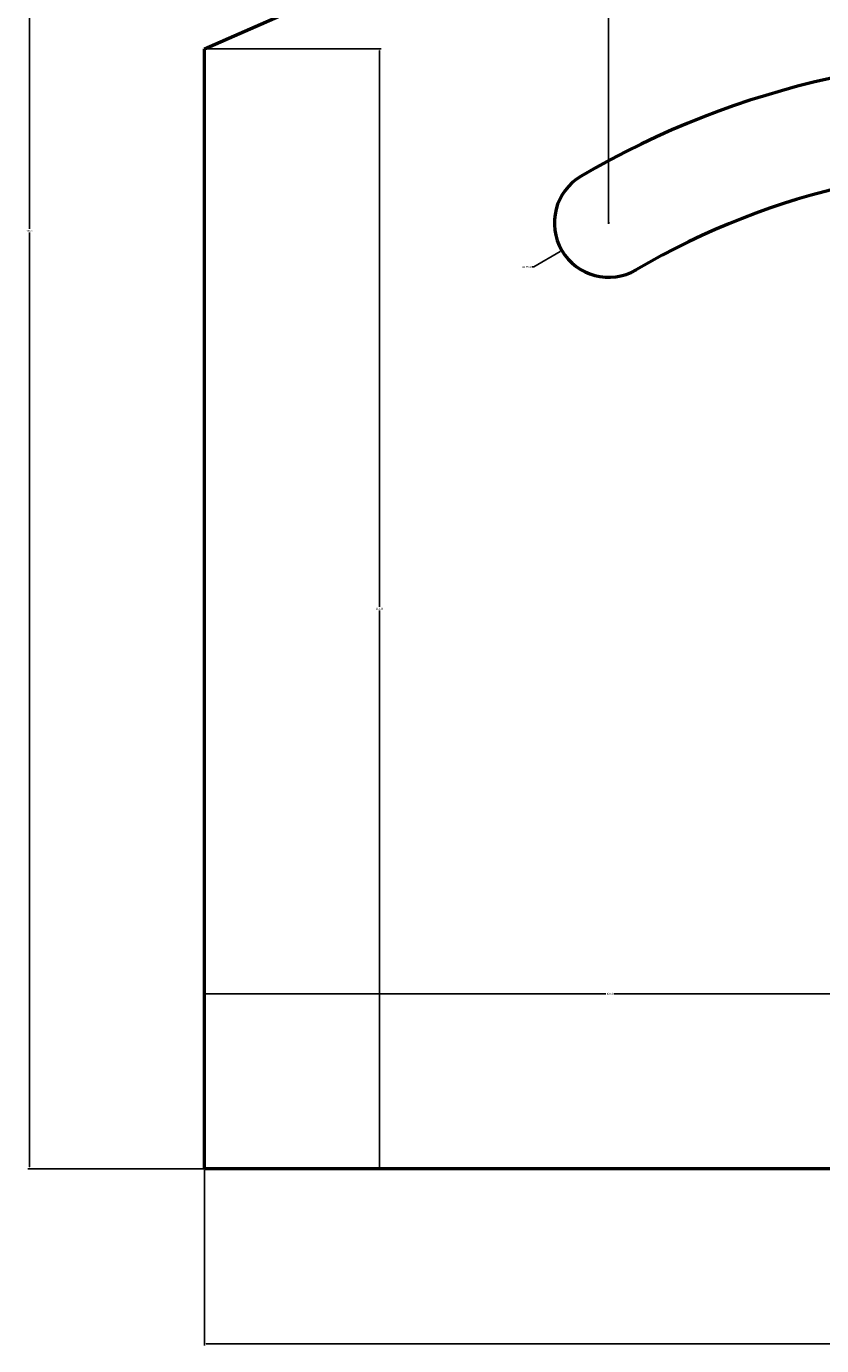
# Model space of a CAD drawing. Units: inches. Extents: x 457 to 775, y 319 to 541.
# Tile 1 of 12: x 457 to 536, y 319 to 450. Entities that reach past the tile are written whole.
import ezdxf

# ---------------------------------------------------------------- set-up
doc = ezdxf.new("R2010")
doc.units = ezdxf.units.IN
doc.header["$MEASUREMENT"] = 0
doc.layers.add('M-DIMS', color=2, linetype='Continuous', lineweight=18)
doc.layers.add('M-OUTL', color=7, linetype='Continuous', lineweight=50)
doc.styles.get("Standard").update_dxf_attribs({"font": 'arial.ttf'})
doc.dimstyles.get("Standard").update_dxf_attribs({"dimtxt": 0.18, "dimasz": 0.18, "dimexe": 0.18, "dimexo": 0.0625, "dimgap": 0.09, "dimtad": 0, "dimtih": 1, "dimtoh": 1, "dimdec": 4, "dimzin": 0, "dimdsep": 46, "dimtxsty": 'Standard', "dimcen": 0.09, "dimadec": 0, "dimazin": 0, "dimtfac": 1, "dimtdec": 4, "dimtofl": 0, "dimtmove": 0, "dimatfit": 3, "dimfxl": 1, "dimtolj": 1, "dimtzin": 0, "dimarcsym": 0})

# ---------------------------------------------------------------- blocks, each defined once
blk = doc.blocks.new('*D2')
at = {"layer": 'Defpoints', "color": 0, "transparency": 16777216}
for p in [(756.93, 375.7), (474.31, 336.7), (756.93, 319.3)]:
    blk.add_point(p, dxfattribs=at)
at = {"layer": 'M-DIMS', "color": 0, "lineweight": -2, "transparency": 16777216}
for p, q in [((756.93, 375.63), (756.93, 319.12)), ((474.31, 336.63), (474.31, 319.12)), ((474.49, 319.3), (615.22, 319.3)), ((756.75, 319.3), (616.01, 319.3))]:
    blk.add_line(p, q, dxfattribs=at)
at = {"layer": 'M-DIMS', "color": 0, "transparency": 16777216}
for points in [[(474.49, 319.33), (474.49, 319.27), (474.31, 319.3)], [(756.75, 319.33), (756.75, 319.27), (756.93, 319.3)]]:
    blk.add_solid(points, dxfattribs=at)
at = {"layer": 'M-DIMS', "color": 0, "transparency": 16777216, "insert": (615.62, 319.3), "char_height": 0.18, "attachment_point": 5}
blk.add_mtext('\\A1;282.6', dxfattribs=at)
blk = doc.blocks.new('*D3')
at = {"layer": 'Defpoints', "color": 0, "transparency": 16777216}
for p in [(456.91, 523.21), (646, 523.21), (474.31, 336.7)]:
    blk.add_point(p, dxfattribs=at)
at = {"layer": 'M-DIMS', "color": 0, "lineweight": -2, "transparency": 16777216}
for p, q in [((645.94, 523.21), (456.73, 523.21)), ((456.91, 523.03), (456.91, 430.14)), ((456.91, 336.88), (456.91, 429.77)), ((474.24, 336.7), (456.73, 336.7))]:
    blk.add_line(p, q, dxfattribs=at)
at = {"layer": 'M-DIMS', "color": 0, "transparency": 16777216}
for points in [[(456.88, 523.03), (456.94, 523.03), (456.91, 523.21)], [(456.88, 336.88), (456.94, 336.88), (456.91, 336.7)]]:
    blk.add_solid(points, dxfattribs=at)
at = {"layer": 'M-DIMS', "color": 0, "transparency": 16777216, "insert": (456.91, 429.95), "char_height": 0.18, "attachment_point": 5}
blk.add_mtext('\\A1;186.5', dxfattribs=at)
blk = doc.blocks.new('*D5')
at = {"layer": 'Defpoints', "color": 0, "transparency": 16777216}
for p in [(474.31, 448.06), (474.31, 336.7), (491.71, 336.7)]:
    blk.add_point(p, dxfattribs=at)
at = {"layer": 'M-DIMS', "color": 0, "lineweight": -2, "transparency": 16777216}
for p, q in [((474.37, 448.06), (491.89, 448.06)), ((491.71, 447.88), (491.71, 392.56)), ((491.71, 336.88), (491.71, 392.2)), ((474.37, 336.7), (491.89, 336.7))]:
    blk.add_line(p, q, dxfattribs=at)
at = {"layer": 'M-DIMS', "color": 0, "transparency": 16777216}
for points in [[(491.68, 447.88), (491.74, 447.88), (491.71, 448.06)], [(491.68, 336.88), (491.74, 336.88), (491.71, 336.7)]]:
    blk.add_solid(points, dxfattribs=at)
at = {"layer": 'M-DIMS', "color": 0, "transparency": 16777216, "insert": (491.71, 392.38), "char_height": 0.18, "attachment_point": 5}
blk.add_mtext('\\A1;111.36', dxfattribs=at)
blk = doc.blocks.new('*D6')
at = {"layer": 'Defpoints', "color": 0, "transparency": 16777216}
for p in [(554.93, 354.1), (474.31, 336.7), (554.93, 336.7)]:
    blk.add_point(p, dxfattribs=at)
at = {"layer": 'M-DIMS', "color": 0, "lineweight": -2, "transparency": 16777216}
for p, q in [((474.31, 336.76), (474.31, 354.28)), ((554.93, 336.76), (554.93, 354.28)), ((474.49, 354.1), (514.23, 354.1)), ((554.75, 354.1), (515.01, 354.1))]:
    blk.add_line(p, q, dxfattribs=at)
at = {"layer": 'M-DIMS', "color": 0, "transparency": 16777216}
for points in [[(474.49, 354.13), (474.49, 354.07), (474.31, 354.1)], [(554.75, 354.13), (554.75, 354.07), (554.93, 354.1)]]:
    blk.add_solid(points, dxfattribs=at)
at = {"layer": 'M-DIMS', "color": 0, "transparency": 16777216, "insert": (514.62, 354.1), "char_height": 0.18, "attachment_point": 5}
blk.add_mtext('\\A1;80.62', dxfattribs=at)
blk = doc.blocks.new('*D16')
at = {"layer": 'Defpoints', "color": 0, "transparency": 16777216}
for p in [(554.93, 540.61), (514.5, 430.73), (554.93, 361.7)]:
    blk.add_point(p, dxfattribs=at)
at = {"layer": 'M-DIMS', "color": 0, "lineweight": -2, "transparency": 16777216}
for p, q in [((514.5, 430.79), (514.5, 540.79)), ((514.68, 540.61), (534.32, 540.61)), ((554.75, 540.61), (535.11, 540.61)), ((554.93, 361.76), (554.93, 540.79))]:
    blk.add_line(p, q, dxfattribs=at)
at = {"layer": 'M-DIMS', "color": 0, "transparency": 16777216}
for points in [[(514.68, 540.64), (514.68, 540.58), (514.5, 540.61)], [(554.75, 540.64), (554.75, 540.58), (554.93, 540.61)]]:
    blk.add_solid(points, dxfattribs=at)
at = {"layer": 'M-DIMS', "color": 0, "transparency": 16777216, "insert": (534.72, 540.61), "char_height": 0.18, "attachment_point": 5}
blk.add_mtext('\\A1;40.43', dxfattribs=at)
blk = doc.blocks.new('*D21')
at = {"layer": 'Defpoints', "color": 0, "transparency": 16777216}
for p in [(514.5, 430.73), (509.84, 428)]:
    blk.add_point(p, dxfattribs=at)
at = {"layer": 'M-DIMS', "color": 0, "lineweight": -2, "transparency": 16777216}
for p, q in [((514.41, 430.73), (514.59, 430.73)), ((514.5, 430.64), (514.5, 430.82)), ((507.05, 426.36), (509.69, 427.91)), ((506.87, 426.36), (507.05, 426.36))]:
    blk.add_line(p, q, dxfattribs=at)
at = {"layer": 'M-DIMS', "color": 0, "transparency": 16777216}
blk.add_solid([(509.67, 427.93), (509.7, 427.88), (509.84, 428)], dxfattribs=at)
at = {"layer": 'M-DIMS', "color": 0, "transparency": 16777216, "insert": (506.33, 426.36), "char_height": 0.18, "attachment_point": 5}
blk.add_mtext('\\A1;2X R5.4', dxfattribs=at)

msp = doc.modelspace()

# ---------------------------------------------------------------- linework, layer by layer
at = {"layer": 'M-OUTL'}
for p, q in [((474.306, 448.059), (646.001, 523.213)), ((474.306, 336.696), (474.306, 448.059)), ((554.931, 336.696), (474.306, 336.696))]:
    msp.add_line(p, q, dxfattribs=at)
for centre, radius, start, end in [((554.931, 361.696), 85.4, 49.61848, 120.35555), ((554.931, 361.696), 74.6, 49.61848, 120.35555), ((514.502, 430.729), 5.4, 120.35555, 300.35555)]:
    msp.add_arc(centre, radius, start, end, dxfattribs=at)

# ---------------------------------------------------------------- dimensions: what is measured, and where the dimension line sits
at = {"layer": 'M-DIMS'}
for base, p1, p2, override, picture, middle in [((554.931, 540.613), (514.502, 430.729), (554.931, 361.696), {"dimdec": 2, "dimlfac": 1, "dimrnd": 0, "dimzin": 0, "dimdsep": 46, "dimlunit": 2}, '*D16', (534.716, 540.613)), ((756.931, 319.296), (474.306, 336.696), (756.931, 375.696), {"dimdec": 1, "dimlfac": 1, "dimrnd": 0, "dimzin": 0, "dimdsep": 46, "dimlunit": 2}, '*D2', (615.619, 319.296)), ((554.931, 354.096), (474.3061, 336.696), (554.931, 336.696), {"dimdec": 2, "dimlfac": 1, "dimrnd": 0, "dimzin": 0, "dimdsep": 46, "dimlunit": 2}, '*D6', (514.6186, 354.096))]:
    dim = msp.add_linear_dim(base=base, p1=p1, p2=p2, dimstyle='Standard', override=override, dxfattribs=at)
    dim.commit()
    dim.dimension.update_dxf_attribs({"geometry": picture, "text_midpoint": middle})
for base, p1, p2, angle, override, picture, middle in [((456.906, 523.213), (474.306, 336.696), (646.001, 523.213), 90, {"dimdec": 1, "dimlfac": 1, "dimrnd": 0, "dimzin": 0, "dimdsep": 46, "dimlunit": 2}, '*D3', (456.906, 429.954)), ((491.706, 336.696), (474.306, 448.059), (474.306, 336.696), 270, {"dimdec": 2, "dimlfac": 1, "dimrnd": 0, "dimzin": 0, "dimdsep": 46, "dimlunit": 2}, '*D5', (491.706, 392.377))]:
    dim = msp.add_linear_dim(base=base, p1=p1, p2=p2, angle=angle, dimstyle='Standard', override=override, dxfattribs=at)
    dim.commit()
    dim.dimension.update_dxf_attribs({"geometry": picture, "text_midpoint": middle})
dim = msp.add_radius_dim(center=(514.502, 430.729), mpoint=(509.842, 428), text='2X <>', dimstyle='Standard', override={"dimdec": 1, "dimlfac": 1, "dimrnd": 0, "dimzin": 0, "dimdsep": 46, "dimlunit": 2}, dxfattribs=at)
dim.commit()
dim.dimension.update_dxf_attribs({"geometry": '*D21', "text_midpoint": (506.331, 426.363), "dimtype": 164})

doc.saveas('drawing.dxf')
